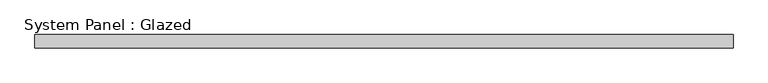
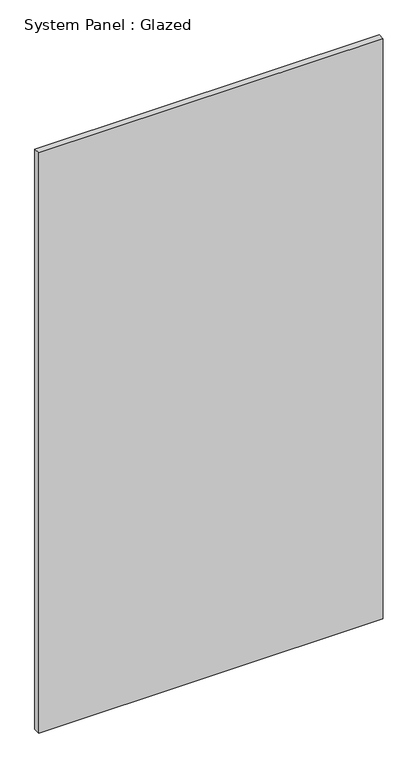
"""IFC4 building model written with IfcOpenShell, lengths in millimetres: plate geometry, System Panel : Glazed."""

from ifc_helpers import new_model, si_unit, origin, origin_with_axes, place, context, project, spatial, polyline, outline, extrude, source, transform, mapped, element, save


def system_panel_glazed_701ad94b(model_context):
    return source(origin(), model_context, "Body", "SweptSolid", [
        extrude(outline(polyline([(667.2791666, 19.05), (-667.2791666, 19.05), (-667.2791666, 44.45), (667.2791666, 44.45), (667.2791666, 19.05)])), origin_with_axes(), (0.0, 0.0, 1.0), 2374.9),
    ])


if __name__ == "__main__":
    model = new_model("IFC4")
    model_context = context("Model", 3, world=origin())
    ifc_project = project(units=[si_unit("LENGTHUNIT", "METRE", prefix="MILLI")], contexts=[model_context])
    site = spatial("IfcSite", under=ifc_project)
    building = spatial("IfcBuilding", under=site)
    placement = place(None, origin())
    system_panel_glazed_shape = system_panel_glazed_701ad94b(model_context)
    element("IfcPlate", 1, ObjectType="System Panel : Glazed", at=placement, inside=building, context=model_context, shape_type="MappedRepresentation", body=[
        mapped(system_panel_glazed_shape, transform((0.0, 0.0, 0.0), x_axis=(1.0, 0.0, 0.0), y_axis=(0.0, 1.0, 0.0), z_axis=(0.0, 0.0, 1.0))),
    ])
    save(model, "model.ifc")

# Revit data of these elements
# Type "System Panel : Glazed"
#   Construction Type Id = "GSP4R"
#   Analytic Construction = "1/8 in Pilkington single glazing"
#   Visual Light Transmittance = 0.9
#   Solar Heat Gain Coefficient = 0.86
#   Heat Transfer Coefficient (U) = 1.18115 BTU/(h·ft²·°F)
#   Define Thermal Properties by = 1
# Element 1 (IfcPlate, "System Panel : Glazed")
#   Materials on its faces: "Glass"
# Materials
#   "Glass": class "Glass", colour RGB 0 128 192, transparency 0.75, Description = "Soda Lime Glass", Cost = 0
